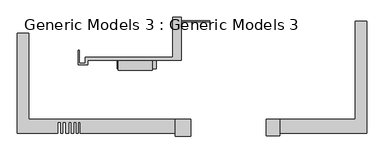
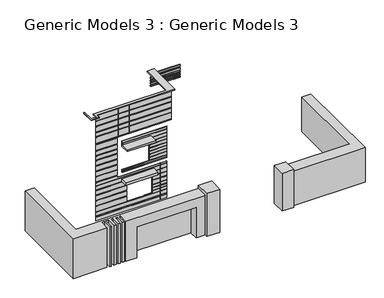
"""IFC4 building model written with IfcOpenShell, lengths in millimetres: proxy geometry, Generic Models 3 : Generic Models 3."""

from ifc_helpers import new_model, si_unit, frame, origin, place, context, project, spatial, polyline, outline, extrude, faceted_brep, source, transform, mapped, element, save


def generic_models_3_generic_models_3_b56d3d43(model_context):
    return source(origin(), model_context, "Body", "SolidModel", [
        faceted_brep([(-6055.6628107, -17805.3512614, 2871.3721498), (-6055.6628107, -17805.3512614, -304.8), (-6055.6628107, -18881.8911988, -304.8), (-6055.6628107, -18881.8911988, 2871.3721498), (-5141.2628107, -17805.3512614, 2871.3721498), (-5141.2628107, -18881.8911988, 2871.3721498), (-5141.2628107, -18881.8911988, -304.8), (-5141.2628107, -18719.7512614, -304.8), (-5141.2628107, -18719.7512614, 2606.1461296), (-5141.2628107, -17805.3512614, 2606.1461296), (-116.9337286, -17805.3512614, 2606.1461296), (-116.9337286, -17805.3512614, -304.8), (-116.9337286, -11273.8752636, -304.8), (619.6662714, -11273.8752636, -304.8), (619.6662714, -18719.7512614, -304.8), (619.6662714, -18719.7512614, 2606.1461296), (619.6662714, -11273.8752636, 2606.1461296), (-116.9337286, -11273.8752636, 2606.1461296)], [[[0, 1, 2, 3]], [[4, 5, 6, 7, 8, 9]], [[1, 0, 4, 9, 10, 11]], [[2, 1, 11, 12, 13, 14, 7, 6]], [[3, 2, 6, 5]], [[0, 3, 5, 4]], [[8, 7, 14, 15]], [[8, 15, 16, 17, 10, 9]], [[15, 14, 13, 16]], [[17, 12, 11, 10]], [[16, 13, 12, 17]]]),
        faceted_brep([(-12088.1628107, -18719.7512614, -304.8), (-12088.1628107, -18719.7512614, 3048.0), (-18387.6766205, -18719.7512614, 3048.0), (-18387.6766205, -18719.7512614, -304.8), (-17520.4293605, -18719.7512614, -304.8), (-17520.4293605, -18719.7512614, 2286.0), (-12796.0293605, -18719.7512614, 2286.0), (-12796.0293605, -18719.7512614, -304.8), (-19348.1660138, -18719.7512614, -304.8), (-19158.4539587, -18719.7512614, -304.8), (-19158.4539587, -18719.7512614, 3048.0), (-19348.1660138, -18719.7512614, 3048.0), (-18980.5989071, -18719.7512614, -304.8), (-18817.6939903, -18719.7512614, -304.8), (-18817.6939903, -18719.7512614, 3048.0), (-18980.5989071, -18719.7512614, 3048.0), (-18661.5366605, -18719.7512614, -304.8), (-18527.0628107, -18719.7512614, -304.8), (-18527.0628107, -18719.7512614, 3048.0), (-18661.5366605, -18719.7512614, 3048.0), (-19674.1502868, -18719.7512614, -304.8), (-19538.6191315, -18719.7512614, -304.8), (-19538.6191315, -18719.7512614, 3048.0), (-19674.1502868, -18719.7512614, 3048.0), (-19887.5763487, -18719.7512614, -304.8), (-19887.5763487, -18719.7512614, 3048.0), (-22558.2115964, -18719.7512614, 3048.0), (-22558.2115964, -18719.7512614, -304.8), (-21821.6115964, -17805.3512614, 3048.0), (-12088.1628107, -17805.3512614, 3048.0), (-12088.1628107, -17805.3512614, 3309.3786493), (-11046.7628107, -17805.3512614, 3309.3786493), (-11046.7628107, -17805.3512614, -304.8), (-21821.6115964, -17805.3512614, -304.8), (-11046.7628107, -18921.6642965, -304.8), (-12088.1628107, -18921.6642965, -304.8), (-12796.0293605, -17983.1512614, -304.8), (-17520.4293605, -17983.1512614, -304.8), (-18387.6766205, -17983.1512614, -304.8), (-18527.0628107, -17983.1512614, -304.8), (-18661.5366605, -17983.1512614, -304.8), (-18817.6939903, -17983.1512614, -304.8), (-18980.5989071, -17983.1512614, -304.8), (-19158.4539587, -17983.1512614, -304.8), (-19348.1660138, -17983.1512614, -304.8), (-19538.6191315, -17983.1512614, -304.8), (-19674.1502868, -17983.1512614, -304.8), (-19887.5763487, -17983.1512614, -304.8), (-22558.2115964, -12082.7142965, -304.8), (-21821.6115964, -12082.7142965, -304.8), (-21821.6115964, -12082.7142965, 3048.0), (-22558.2115964, -12082.7142965, 3048.0), (-19887.5763487, -17983.1512614, 3048.0), (-19674.1502868, -17983.1512614, 3048.0), (-19538.6191315, -17983.1512614, 3048.0), (-19348.1660138, -17983.1512614, 3048.0), (-19158.4539587, -17983.1512614, 3048.0), (-18980.5989071, -17983.1512614, 3048.0), (-18817.6939903, -17983.1512614, 3048.0), (-18661.5366605, -17983.1512614, 3048.0), (-18527.0628107, -17983.1512614, 3048.0), (-18387.6766205, -17983.1512614, 3048.0), (-11046.7628107, -18921.6642965, 3309.3786493), (-12088.1628107, -18921.6642965, 3309.3786493), (-17520.4293605, -17983.1512614, 2286.0), (-12796.0293605, -17983.1512614, 2286.0)], [[[0, 1, 2, 3, 4, 5, 6, 7]], [[8, 9, 10, 11]], [[12, 13, 14, 15]], [[16, 17, 18, 19]], [[20, 21, 22, 23]], [[24, 25, 26, 27]], [[28, 29, 30, 31, 32, 33]], [[32, 34, 35, 0, 7, 36, 37, 4, 3, 38, 39, 17, 16, 40, 41, 13, 12, 42, 43, 9, 8, 44, 45, 21, 20, 46, 47, 24, 27, 48, 49, 33]], [[29, 28, 50, 51, 26, 25, 52, 53, 23, 22, 54, 55, 11, 10, 56, 57, 15, 14, 58, 59, 19, 18, 60, 61, 2, 1]], [[62, 34, 32, 31]], [[63, 30, 29, 1, 0, 35]], [[34, 62, 63, 35]], [[62, 31, 30, 63]], [[44, 55, 54, 45]], [[42, 57, 56, 43]], [[40, 59, 58, 41]], [[38, 61, 60, 39]], [[46, 53, 52, 47]], [[45, 54, 22, 21]], [[55, 44, 8, 11]], [[43, 56, 10, 9]], [[57, 42, 12, 15]], [[41, 58, 14, 13]], [[59, 40, 16, 19]], [[39, 60, 18, 17]], [[61, 38, 3, 2]], [[47, 52, 25, 24]], [[53, 46, 20, 23]], [[64, 37, 36, 65]], [[64, 65, 6, 5]], [[65, 36, 7, 6]], [[37, 64, 5, 4]], [[51, 48, 27, 26]], [[49, 50, 28, 33]], [[48, 51, 50, 49]]]),
        faceted_brep([(-13612.1628107, -13816.2642965, 5651.3031317), (-15860.0628107, -13816.2642965, 5651.3031317), (-15860.0628107, -14540.4385796, 5651.3031317), (-13612.1628107, -14540.4385796, 5651.3031317), (-13612.1628107, -14540.4385796, 5498.9031317), (-15860.0628107, -14540.4385796, 5498.9031317), (-15860.0628107, -13816.2642965, 5498.9031317), (-13612.1628107, -13816.2642965, 5498.9031317), (-13612.1628107, -13841.6642965, 5498.9031317), (-13612.1628107, -13867.0642965, 5498.9031317)], [[[0, 1, 2, 3]], [[4, 5, 6, 7, 8, 9]], [[1, 0, 7, 6]], [[2, 1, 6, 5]], [[3, 2, 5, 4]], [[0, 3, 4, 9, 8, 7]]]),
        faceted_brep([(-15923.5628107, -13867.0642965, 2606.1461296), (-15923.5628107, -13867.0642965, 2821.2917707), (-13354.9773607, -13867.0642965, 2821.2917707), (-13354.9773607, -13867.0642965, 2606.1461296), (-12316.7628107, -13867.0642965, 2606.1461296), (-12316.7628107, -13867.0642965, 2882.1098353), (-17960.2455482, -13867.0642965, 2882.1098353), (-17960.2455482, -13867.0642965, 2606.1461296), (-12316.7628107, -13867.0642965, 3048.0), (-16279.1628107, -13867.0642965, 3048.0), (-16279.1628107, -13867.0642965, 3184.518053), (-17960.2455482, -13867.0642965, 3184.518053), (-17960.2455482, -13867.0642965, 2942.2726161), (-12316.7628107, -13867.0642965, 2942.2726161), (-17960.2455482, -13867.0642965, 0.0), (-12316.7628107, -13867.0642965, 0.0), (-12316.7628107, -13867.0642965, 304.8), (-17960.2455482, -13867.0642965, 304.8), (-11973.8628107, -13867.0642965, 8818.1896751), (-17960.2455482, -13867.0642965, 8818.1896751), (-17960.2455482, -13867.0642965, 8418.5654464), (-11973.8628107, -13867.0642965, 8418.5654464), (-15517.1628107, -13867.0642965, 2175.1008614), (-15517.1628107, -13867.0642965, 2535.4608087), (-17960.2455482, -13867.0642965, 2535.4608087), (-17960.2455482, -13867.0642965, 2175.1008614), (-15517.1628107, -13867.0642965, 1735.9125615), (-15517.1628107, -13867.0642965, 2120.9543587), (-17960.2455482, -13867.0642965, 2120.9543587), (-17960.2455482, -13867.0642965, 1735.9125615), (-15517.1628107, -13867.0642965, 763.0716334), (-15517.1628107, -13867.0642965, 1206.4800905), (-17960.2455482, -13867.0642965, 1206.4800905), (-17960.2455482, -13867.0642965, 763.0716334), (-15517.1628107, -13867.0642965, 1266.6428713), (-15517.1628107, -13867.0642965, 1684.6088815), (-17960.2455482, -13867.0642965, 1684.6088815), (-17960.2455482, -13867.0642965, 1266.6428713), (-12316.7628107, -13867.0642965, 400.2988277), (-12316.7628107, -13867.0642965, 695.0964536), (-17960.2455482, -13867.0642965, 695.0964536), (-17960.2455482, -13867.0642965, 400.2988277), (-16279.1628107, -13867.0642965, 5917.4274118), (-16279.1628107, -13867.0642965, 6400.8), (-17960.2455482, -13867.0642965, 6400.8), (-17960.2455482, -13867.0642965, 5917.4274118), (-16279.1628107, -13867.0642965, 5498.9031317), (-16279.1628107, -13867.0642965, 5825.6641304), (-17960.2455482, -13867.0642965, 5825.6641304), (-17960.2455482, -13867.0642965, 5498.9031317), (-16279.1628107, -13867.0642965, 5103.7107607), (-16279.1628107, -13867.0642965, 5410.5409428), (-17960.2455482, -13867.0642965, 5410.5409428), (-17960.2455482, -13867.0642965, 5103.7107607), (-16279.1628107, -13867.0642965, 4670.5387389), (-16279.1628107, -13867.0642965, 5043.5479799), (-17960.2455482, -13867.0642965, 5043.5479799), (-17960.2455482, -13867.0642965, 4670.5387389), (-16279.1628107, -13867.0642965, 4207.2853267), (-16279.1628107, -13867.0642965, 4598.343402), (-17960.2455482, -13867.0642965, 4598.343402), (-17960.2455482, -13867.0642965, 4207.2853267), (-16279.1628107, -13867.0642965, 3750.0481926), (-16279.1628107, -13867.0642965, 4124.9991955), (-17960.2455482, -13867.0642965, 4124.9991955), (-17960.2455482, -13867.0642965, 3750.0481926), (-16279.1628107, -13867.0642965, 3256.71339), (-16279.1628107, -13867.0642965, 3701.917968), (-17960.2455482, -13867.0642965, 3701.917968), (-17960.2455482, -13867.0642965, 3256.71339), (-11973.8628107, -13867.0642965, 7978.3125268), (-11973.8628107, -13867.0642965, 8337.4712494), (-17960.2455482, -13867.0642965, 8337.4712494), (-17960.2455482, -13867.0642965, 7978.3125268), (-11973.8628107, -13867.0642965, 7494.0021413), (-11973.8628107, -13867.0642965, 7895.2878893), (-17960.2455482, -13867.0642965, 7895.2878893), (-17960.2455482, -13867.0642965, 7494.0021413), (-11973.8628107, -13867.0642965, 7078.8789538), (-11973.8628107, -13867.0642965, 7410.9775038), (-17960.2455482, -13867.0642965, 7410.9775038), (-17960.2455482, -13867.0642965, 7078.8789538), (-11973.8628107, -13867.0642965, 6495.9664367), (-11973.8628107, -13867.0642965, 7011.586349), (-17960.2455482, -13867.0642965, 7011.586349), (-17960.2455482, -13867.0642965, 6495.9664367), (-13497.8628107, -13867.0642965, 763.0716334), (-12316.7628107, -13867.0642965, 763.0716334), (-12316.7628107, -13867.0642965, 953.616846), (-13497.8628107, -13867.0642965, 953.616846), (-13497.8628107, -13867.0642965, 2540.7233827), (-13497.8628107, -13867.0642965, 2245.0272955), (-12316.7628107, -13867.0642965, 2245.0272955), (-12316.7628107, -13867.0642965, 2540.7233827), (-13497.8628107, -13867.0642965, 2176.789737), (-13497.8628107, -13867.0642965, 1876.5444793), (-12316.7628107, -13867.0642965, 1876.5444793), (-12316.7628107, -13867.0642965, 2176.789737), (-13497.8628107, -13867.0642965, 1822.5907344), (-13497.8628107, -13867.0642965, 1524.0), (-12316.7628107, -13867.0642965, 1524.0), (-12316.7628107, -13867.0642965, 1822.5907344), (-13497.8628107, -13867.0642965, 1462.5699573), (-13497.8628107, -13867.0642965, 1249.7277266), (-12316.7628107, -13867.0642965, 1249.7277266), (-12316.7628107, -13867.0642965, 1462.5699573), (-13497.8628107, -13867.0642965, 1194.1688936), (-13497.8628107, -13867.0642965, 1001.3322189), (-12316.7628107, -13867.0642965, 1001.3322189), (-12316.7628107, -13867.0642965, 1194.1688936), (-15923.5628107, -13816.2642965, 2606.1461296), (-15517.1628107, -13816.2642965, 2606.1461296), (-15517.1628107, -13816.2642965, 0.0), (-16170.5880908, -13816.2642965, 0.0), (-16170.5880908, -13816.2642965, 3048.0), (-12953.063671, -13816.2642965, 3048.0), (-12953.063671, -13816.2642965, 0.0), (-13497.8628107, -13816.2642965, 0.0), (-13497.8628107, -13816.2642965, 2606.1461296), (-13354.9773607, -13816.2642965, 2606.1461296), (-13354.9773607, -13816.2642965, 2821.2917707), (-15923.5628107, -13816.2642965, 2821.2917707), (-12316.7628107, -13816.2642965, 3048.0), (-12316.7628107, -13816.2642965, 0.0), (-12850.1628107, -13816.2642965, 0.0), (-12850.1628107, -13816.2642965, 3048.0), (-11973.8628107, -13816.2642965, 8818.1896751), (-11973.8628107, -13816.2642965, 6400.8), (-12768.5357054, -13816.2642965, 6400.8), (-12768.5357054, -13816.2642965, 8818.1896751), (-17960.2455482, -13816.2642965, 0.0), (-17960.2455482, -13816.2642965, 8818.1896751), (-17079.2628107, -13816.2642965, 8818.1896751), (-17079.2628107, -13816.2642965, 0.0), (-16279.1628107, -13816.2642965, 0.0), (-16980.0783065, -13816.2642965, 0.0), (-16980.0783065, -13816.2642965, 8818.1896751), (-16279.1628107, -13816.2642965, 8818.1896751), (-14673.1364765, -13816.2642965, 0.0), (-15421.9128107, -13816.2642965, 0.0), (-15421.9128107, -13816.2642965, 763.0716334), (-14673.1364765, -13816.2642965, 763.0716334), (-13565.9475269, -13816.2642965, 0.0), (-14032.5674721, -13816.2642965, 0.0), (-14032.5674721, -13816.2642965, 763.0716334), (-13565.9475269, -13816.2642965, 763.0716334), (-14071.4524675, -13816.2642965, 0.0), (-14564.6628107, -13816.2642965, 0.0), (-14564.6628107, -13816.2642965, 763.0716334), (-14071.4524675, -13816.2642965, 763.0716334), (-16187.9466003, -13816.2642965, 8818.1896751), (-15402.8628107, -13816.2642965, 8818.1896751), (-15402.8628107, -13816.2642965, 6495.9664367), (-15312.895459, -13816.2642965, 6495.9664367), (-15312.895459, -13816.2642965, 8818.1896751), (-14567.4028515, -13816.2642965, 8818.1896751), (-14567.4028515, -13816.2642965, 6400.8), (-16187.9466003, -13816.2642965, 6400.8), (-14463.6220546, -13816.2642965, 8818.1896751), (-13726.4628107, -13816.2642965, 8818.1896751), (-13726.4628107, -13816.2642965, 6400.8), (-14463.6220546, -13816.2642965, 6400.8), (-13612.1628107, -13816.2642965, 8818.1896751), (-12879.2352221, -13816.2642965, 8818.1896751), (-12879.2352221, -13816.2642965, 6400.8), (-13612.1628107, -13816.2642965, 6400.8), (-17960.2455482, -13841.6642965, 304.8), (-17960.2455482, -13841.6642965, 400.2988277), (-17960.2455482, -13841.6642965, 695.0964536), (-17960.2455482, -13841.6642965, 763.0716334), (-17960.2455482, -13841.6642965, 1206.4800905), (-17960.2455482, -13841.6642965, 1266.6428713), (-17960.2455482, -13841.6642965, 1684.6088815), (-17960.2455482, -13841.6642965, 1735.9125615), (-17960.2455482, -13841.6642965, 2120.9543587), (-17960.2455482, -13841.6642965, 2175.1008614), (-17960.2455482, -13841.6642965, 2535.4608087), (-17960.2455482, -13841.6642965, 2606.1461296), (-17960.2455482, -13841.6642965, 2882.1098353), (-17960.2455482, -13841.6642965, 2942.2726161), (-17960.2455482, -13841.6642965, 3184.518053), (-17960.2455482, -13841.6642965, 3256.71339), (-17960.2455482, -13841.6642965, 3701.917968), (-17960.2455482, -13841.6642965, 3750.0481926), (-17960.2455482, -13841.6642965, 4124.9991955), (-17960.2455482, -13841.6642965, 4207.2853267), (-17960.2455482, -13841.6642965, 4598.343402), (-17960.2455482, -13841.6642965, 4670.5387389), (-17960.2455482, -13841.6642965, 5043.5479799), (-17960.2455482, -13841.6642965, 5103.7107607), (-17960.2455482, -13841.6642965, 5410.5409428), (-17960.2455482, -13841.6642965, 5498.9031317), (-17960.2455482, -13841.6642965, 5825.6641304), (-17960.2455482, -13841.6642965, 5917.4274118), (-17960.2455482, -13841.6642965, 6400.8), (-17960.2455482, -13841.6642965, 6495.9664367), (-17960.2455482, -13841.6642965, 7011.586349), (-17960.2455482, -13841.6642965, 7078.8789538), (-17960.2455482, -13841.6642965, 7410.9775038), (-17960.2455482, -13841.6642965, 7494.0021413), (-17960.2455482, -13841.6642965, 7895.2878893), (-17960.2455482, -13841.6642965, 7978.3125268), (-17960.2455482, -13841.6642965, 8337.4712494), (-17960.2455482, -13841.6642965, 8418.5654464), (-17079.2628107, -13841.6642965, 0.0), (-16980.0783065, -13841.6642965, 0.0), (-16279.1628107, -13841.6642965, 0.0), (-16170.5880908, -13841.6642965, 0.0), (-15517.1628107, -13841.6642965, 0.0), (-15421.9128107, -13841.6642965, 0.0), (-14673.1364765, -13841.6642965, 0.0), (-14564.6628107, -13841.6642965, 0.0), (-14071.4524675, -13841.6642965, 0.0), (-14032.5674721, -13841.6642965, 0.0), (-13565.9475269, -13841.6642965, 0.0), (-13497.8628107, -13841.6642965, 0.0), (-12953.063671, -13841.6642965, 0.0), (-12850.1628107, -13841.6642965, 0.0), (-16279.1628107, -13841.6642965, 5917.4274118), (-16279.1628107, -13841.6642965, 5825.6641304), (-16279.1628107, -13841.6642965, 5498.9031317), (-16279.1628107, -13841.6642965, 5410.5409428), (-16279.1628107, -13841.6642965, 5103.7107607), (-16279.1628107, -13841.6642965, 5043.5479799), (-16279.1628107, -13841.6642965, 4670.5387389), (-16279.1628107, -13841.6642965, 4598.343402), (-16279.1628107, -13841.6642965, 4207.2853267), (-16279.1628107, -13841.6642965, 4124.9991955), (-16279.1628107, -13841.6642965, 3750.0481926), (-16279.1628107, -13841.6642965, 3701.917968), (-16279.1628107, -13841.6642965, 3256.71339), (-16279.1628107, -13841.6642965, 3184.518053), (-16279.1628107, -13841.6642965, 3048.0), (-16279.1628107, -13841.6642965, 2942.2726161), (-16279.1628107, -13841.6642965, 2882.1098353), (-16279.1628107, -13841.6642965, 2606.1461296), (-16279.1628107, -13841.6642965, 2535.4608087), (-16279.1628107, -13841.6642965, 2175.1008614), (-16279.1628107, -13841.6642965, 2120.9543587), (-16279.1628107, -13841.6642965, 1735.9125615), (-16279.1628107, -13841.6642965, 1684.6088815), (-16279.1628107, -13841.6642965, 1266.6428713), (-16279.1628107, -13841.6642965, 1206.4800905), (-16279.1628107, -13841.6642965, 763.0716334), (-16279.1628107, -13841.6642965, 695.0964536), (-16279.1628107, -13841.6642965, 400.2988277), (-16279.1628107, -13841.6642965, 304.8), (-16279.1628107, -13841.6642965, 8818.1896751), (-16279.1628107, -13841.6642965, 8418.5654464), (-16279.1628107, -13841.6642965, 8337.4712494), (-16279.1628107, -13841.6642965, 7978.3125268), (-16279.1628107, -13841.6642965, 7895.2878893), (-16279.1628107, -13841.6642965, 7494.0021413), (-16279.1628107, -13841.6642965, 7410.9775038), (-16279.1628107, -13841.6642965, 7078.8789538), (-16279.1628107, -13841.6642965, 7011.586349), (-16279.1628107, -13841.6642965, 6495.9664367), (-16279.1628107, -13841.6642965, 6400.8), (-12850.1628107, -13841.6642965, 3048.0), (-12953.063671, -13841.6642965, 3048.0), (-16170.5880908, -13841.6642965, 3048.0), (-15517.1628107, -13841.6642965, 2175.1008614), (-15517.1628107, -13841.6642965, 2120.9543587), (-15517.1628107, -13841.6642965, 1735.9125615), (-15517.1628107, -13841.6642965, 1684.6088815), (-15517.1628107, -13841.6642965, 1266.6428713), (-15517.1628107, -13841.6642965, 1206.4800905), (-15517.1628107, -13841.6642965, 763.0716334), (-15517.1628107, -13841.6642965, 695.0964536), (-15517.1628107, -13841.6642965, 400.2988277), (-15517.1628107, -13841.6642965, 304.8), (-15517.1628107, -13841.6642965, 2606.1461296), (-15517.1628107, -13841.6642965, 2535.4608087), (-13354.9773607, -13701.9642965, 2821.2917707), (-15923.5628107, -13701.9642965, 2821.2917707), (-15923.5628107, -14431.1224926, 2821.2917707), (-13354.9773607, -14431.1224926, 2821.2917707), (-13354.9773607, -14431.1224926, 2606.1461296), (-15923.5628107, -14431.1224926, 2606.1461296), (-17079.2628107, -13841.6642965, 2606.1461296), (-16980.0783065, -13841.6642965, 2606.1461296), (-16170.5880908, -13841.6642965, 2606.1461296), (-15923.5628107, -13701.9642965, 2606.1461296), (-13354.9773607, -13701.9642965, 2606.1461296), (-13497.8628107, -13841.6642965, 2606.1461296), (-12953.063671, -13841.6642965, 2606.1461296), (-12850.1628107, -13841.6642965, 2606.1461296), (-12316.7628107, -13841.6642965, 2606.1461296), (-12316.7628107, -13841.6642965, 2942.2726161), (-12316.7628107, -13841.6642965, 2882.1098353), (-12316.7628107, -13841.6642965, 2540.7233827), (-12316.7628107, -13841.6642965, 2245.0272955), (-12316.7628107, -13841.6642965, 2176.789737), (-12316.7628107, -13841.6642965, 1876.5444793), (-12316.7628107, -13841.6642965, 1822.5907344), (-12316.7628107, -13841.6642965, 1524.0), (-12316.7628107, -13841.6642965, 1462.5699573), (-12316.7628107, -13841.6642965, 1249.7277266), (-12316.7628107, -13841.6642965, 1194.1688936), (-12316.7628107, -13841.6642965, 1001.3322189), (-12316.7628107, -13841.6642965, 953.616846), (-12316.7628107, -13841.6642965, 763.0716334), (-12316.7628107, -13841.6642965, 695.0964536), (-12316.7628107, -13841.6642965, 400.2988277), (-12316.7628107, -13841.6642965, 304.8), (-13497.8628107, -13841.6642965, 763.0716334), (-13497.8628107, -13841.6642965, 953.616846), (-13497.8628107, -13841.6642965, 1001.3322189), (-13497.8628107, -13841.6642965, 1194.1688936), (-13497.8628107, -13841.6642965, 1249.7277266), (-13497.8628107, -13841.6642965, 1462.5699573), (-13497.8628107, -13841.6642965, 1524.0), (-13497.8628107, -13841.6642965, 1822.5907344), (-13497.8628107, -13841.6642965, 1876.5444793), (-13497.8628107, -13841.6642965, 2176.789737), (-13497.8628107, -13841.6642965, 2245.0272955), (-13497.8628107, -13841.6642965, 2540.7233827), (-13497.8628107, -13841.6642965, 304.8), (-13497.8628107, -13841.6642965, 400.2988277), (-13497.8628107, -13841.6642965, 695.0964536), (-15421.9128107, -13841.6642965, 763.0716334), (-14673.1364765, -13841.6642965, 763.0716334), (-14032.5674721, -13841.6642965, 763.0716334), (-13565.9475269, -13841.6642965, 763.0716334), (-14564.6628107, -13841.6642965, 763.0716334), (-14071.4524675, -13841.6642965, 763.0716334), (-11973.8628107, -13841.6642965, 8418.5654464), (-11973.8628107, -13841.6642965, 8337.4712494), (-11973.8628107, -13841.6642965, 7978.3125268), (-11973.8628107, -13841.6642965, 7895.2878893), (-11973.8628107, -13841.6642965, 7494.0021413), (-11973.8628107, -13841.6642965, 7410.9775038), (-11973.8628107, -13841.6642965, 7078.8789538), (-11973.8628107, -13841.6642965, 7011.586349), (-11973.8628107, -13841.6642965, 6495.9664367), (-11973.8628107, -13841.6642965, 6400.8), (-12768.5357054, -13841.6642965, 8818.1896751), (-12879.2352221, -13841.6642965, 8818.1896751), (-13612.1628107, -13841.6642965, 8818.1896751), (-13726.4628107, -13841.6642965, 8818.1896751), (-14463.6220546, -13841.6642965, 8818.1896751), (-14567.4028515, -13841.6642965, 8818.1896751), (-15312.895459, -13841.6642965, 8818.1896751), (-15402.8628107, -13841.6642965, 8818.1896751), (-16187.9466003, -13841.6642965, 8818.1896751), (-16980.0783065, -13841.6642965, 8818.1896751), (-17079.2628107, -13841.6642965, 8818.1896751), (-14567.4028515, -13841.6642965, 6400.8), (-16187.9466003, -13841.6642965, 6400.8), (-13726.4628107, -13841.6642965, 6400.8), (-14463.6220546, -13841.6642965, 6400.8), (-12879.2352221, -13841.6642965, 6400.8), (-13612.1628107, -13841.6642965, 6400.8), (-12768.5357054, -13841.6642965, 6400.8), (-17079.2628107, -13841.6642965, 304.8), (-17079.2628107, -13841.6642965, 400.2988277), (-17079.2628107, -13841.6642965, 695.0964536), (-17079.2628107, -13841.6642965, 763.0716334), (-17079.2628107, -13841.6642965, 1206.4800905), (-17079.2628107, -13841.6642965, 1266.6428713), (-17079.2628107, -13841.6642965, 1684.6088815), (-17079.2628107, -13841.6642965, 1735.9125615), (-17079.2628107, -13841.6642965, 2120.9543587), (-17079.2628107, -13841.6642965, 2175.1008614), (-17079.2628107, -13841.6642965, 2535.4608087), (-17079.2628107, -13841.6642965, 2882.1098353), (-17079.2628107, -13841.6642965, 2942.2726161), (-17079.2628107, -13841.6642965, 3184.518053), (-17079.2628107, -13841.6642965, 3256.71339), (-17079.2628107, -13841.6642965, 3701.917968), (-17079.2628107, -13841.6642965, 3750.0481926), (-17079.2628107, -13841.6642965, 4124.9991955), (-17079.2628107, -13841.6642965, 4207.2853267), (-17079.2628107, -13841.6642965, 4598.343402), (-17079.2628107, -13841.6642965, 4670.5387389), (-17079.2628107, -13841.6642965, 5043.5479799), (-17079.2628107, -13841.6642965, 5103.7107607), (-17079.2628107, -13841.6642965, 5410.5409428), (-17079.2628107, -13841.6642965, 5498.9031317), (-17079.2628107, -13841.6642965, 5825.6641304), (-17079.2628107, -13841.6642965, 5917.4274118), (-17079.2628107, -13841.6642965, 6400.8), (-17079.2628107, -13841.6642965, 6495.9664367), (-17079.2628107, -13841.6642965, 7011.586349), (-17079.2628107, -13841.6642965, 7078.8789538), (-17079.2628107, -13841.6642965, 7410.9775038), (-17079.2628107, -13841.6642965, 7494.0021413), (-17079.2628107, -13841.6642965, 7895.2878893), (-17079.2628107, -13841.6642965, 7978.3125268), (-17079.2628107, -13841.6642965, 8337.4712494), (-17079.2628107, -13841.6642965, 8418.5654464), (-16980.0783065, -13841.6642965, 5917.4274118), (-16980.0783065, -13841.6642965, 5825.6641304), (-16980.0783065, -13841.6642965, 5498.9031317), (-16980.0783065, -13841.6642965, 5410.5409428), (-16980.0783065, -13841.6642965, 5103.7107607), (-16980.0783065, -13841.6642965, 5043.5479799), (-16980.0783065, -13841.6642965, 4670.5387389), (-16980.0783065, -13841.6642965, 4598.343402), (-16980.0783065, -13841.6642965, 4207.2853267), (-16980.0783065, -13841.6642965, 4124.9991955), (-16980.0783065, -13841.6642965, 3750.0481926), (-16980.0783065, -13841.6642965, 3701.917968), (-16980.0783065, -13841.6642965, 3256.71339), (-16980.0783065, -13841.6642965, 3184.518053), (-16170.5880908, -13841.6642965, 2175.1008614), (-16170.5880908, -13841.6642965, 2120.9543587), (-16170.5880908, -13841.6642965, 1735.9125615), (-16170.5880908, -13841.6642965, 1684.6088815), (-16170.5880908, -13841.6642965, 1266.6428713), (-16170.5880908, -13841.6642965, 1206.4800905), (-16170.5880908, -13841.6642965, 2535.4608087), (-16980.0783065, -13841.6642965, 2535.4608087), (-12850.1628107, -13841.6642965, 2942.2726161), (-12850.1628107, -13841.6642965, 2882.1098353), (-12850.1628107, -13841.6642965, 763.0716334), (-12850.1628107, -13841.6642965, 695.0964536), (-12850.1628107, -13841.6642965, 400.2988277), (-12850.1628107, -13841.6642965, 304.8), (-15421.9128107, -13841.6642965, 695.0964536), (-14673.1364765, -13841.6642965, 695.0964536), (-14032.5674721, -13841.6642965, 695.0964536), (-13565.9475269, -13841.6642965, 695.0964536), (-14564.6628107, -13841.6642965, 695.0964536), (-14071.4524675, -13841.6642965, 695.0964536), (-12768.5357054, -13841.6642965, 8418.5654464), (-12768.5357054, -13841.6642965, 8337.4712494), (-12768.5357054, -13841.6642965, 7978.3125268), (-12768.5357054, -13841.6642965, 7895.2878893), (-12768.5357054, -13841.6642965, 7494.0021413), (-12768.5357054, -13841.6642965, 7410.9775038), (-12768.5357054, -13841.6642965, 7078.8789538), (-12768.5357054, -13841.6642965, 7011.586349), (-12768.5357054, -13841.6642965, 6495.9664367), (-14567.4028515, -13841.6642965, 6495.9664367), (-15312.895459, -13841.6642965, 6495.9664367), (-15402.8628107, -13841.6642965, 6495.9664367), (-16187.9466003, -13841.6642965, 6495.9664367), (-13726.4628107, -13841.6642965, 6495.9664367), (-14463.6220546, -13841.6642965, 6495.9664367), (-12879.2352221, -13841.6642965, 6495.9664367), (-13612.1628107, -13841.6642965, 6495.9664367), (-15402.8628107, -13841.6642965, 8418.5654464), (-16187.9466003, -13841.6642965, 8418.5654464), (-16187.9466003, -13841.6642965, 8337.4712494), (-15402.8628107, -13841.6642965, 8337.4712494), (-14567.4028515, -13841.6642965, 8418.5654464), (-15312.895459, -13841.6642965, 8418.5654464), (-15312.895459, -13841.6642965, 8337.4712494), (-14567.4028515, -13841.6642965, 8337.4712494), (-13726.4628107, -13841.6642965, 8418.5654464), (-14463.6220546, -13841.6642965, 8418.5654464), (-14463.6220546, -13841.6642965, 8337.4712494), (-13726.4628107, -13841.6642965, 8337.4712494), (-12879.2352221, -13841.6642965, 8418.5654464), (-13612.1628107, -13841.6642965, 8418.5654464), (-13612.1628107, -13841.6642965, 8337.4712494), (-12879.2352221, -13841.6642965, 8337.4712494), (-16980.0783065, -13841.6642965, 8418.5654464), (-16980.0783065, -13841.6642965, 8337.4712494), (-15402.8628107, -13841.6642965, 7978.3125268), (-16187.9466003, -13841.6642965, 7978.3125268), (-16187.9466003, -13841.6642965, 7895.2878893), (-15402.8628107, -13841.6642965, 7895.2878893), (-14567.4028515, -13841.6642965, 7978.3125268), (-15312.895459, -13841.6642965, 7978.3125268), (-15312.895459, -13841.6642965, 7895.2878893), (-14567.4028515, -13841.6642965, 7895.2878893), (-13726.4628107, -13841.6642965, 7978.3125268), (-14463.6220546, -13841.6642965, 7978.3125268), (-14463.6220546, -13841.6642965, 7895.2878893), (-13726.4628107, -13841.6642965, 7895.2878893), (-12879.2352221, -13841.6642965, 7978.3125268), (-13612.1628107, -13841.6642965, 7978.3125268), (-13612.1628107, -13841.6642965, 7895.2878893), (-12879.2352221, -13841.6642965, 7895.2878893), (-16980.0783065, -13841.6642965, 7978.3125268), (-16980.0783065, -13841.6642965, 7895.2878893), (-15402.8628107, -13841.6642965, 7494.0021413), (-16187.9466003, -13841.6642965, 7494.0021413), (-16187.9466003, -13841.6642965, 7410.9775038), (-15402.8628107, -13841.6642965, 7410.9775038), (-14567.4028515, -13841.6642965, 7494.0021413), (-15312.895459, -13841.6642965, 7494.0021413), (-15312.895459, -13841.6642965, 7410.9775038), (-14567.4028515, -13841.6642965, 7410.9775038), (-13726.4628107, -13841.6642965, 7494.0021413), (-14463.6220546, -13841.6642965, 7494.0021413), (-14463.6220546, -13841.6642965, 7410.9775038), (-13726.4628107, -13841.6642965, 7410.9775038), (-12879.2352221, -13841.6642965, 7494.0021413), (-13612.1628107, -13841.6642965, 7494.0021413), (-13612.1628107, -13841.6642965, 7410.9775038), (-12879.2352221, -13841.6642965, 7410.9775038), (-16980.0783065, -13841.6642965, 7494.0021413), (-16980.0783065, -13841.6642965, 7410.9775038), (-15402.8628107, -13841.6642965, 7078.8789538), (-16187.9466003, -13841.6642965, 7078.8789538), (-16187.9466003, -13841.6642965, 7011.586349), (-15402.8628107, -13841.6642965, 7011.586349), (-14567.4028515, -13841.6642965, 7078.8789538), (-15312.895459, -13841.6642965, 7078.8789538), (-15312.895459, -13841.6642965, 7011.586349), (-14567.4028515, -13841.6642965, 7011.586349), (-13726.4628107, -13841.6642965, 7078.8789538), (-14463.6220546, -13841.6642965, 7078.8789538), (-14463.6220546, -13841.6642965, 7011.586349), (-13726.4628107, -13841.6642965, 7011.586349), (-12879.2352221, -13841.6642965, 7078.8789538), (-13612.1628107, -13841.6642965, 7078.8789538), (-13612.1628107, -13841.6642965, 7011.586349), (-12879.2352221, -13841.6642965, 7011.586349), (-16980.0783065, -13841.6642965, 7078.8789538), (-16980.0783065, -13841.6642965, 7011.586349), (-16980.0783065, -13841.6642965, 6495.9664367), (-16980.0783065, -13841.6642965, 6400.8), (-16980.0783065, -13841.6642965, 2942.2726161), (-16980.0783065, -13841.6642965, 2882.1098353), (-12953.063671, -13841.6642965, 2942.2726161), (-16170.5880908, -13841.6642965, 2942.2726161), (-16170.5880908, -13841.6642965, 2882.1098353), (-12953.063671, -13841.6642965, 2882.1098353), (-16980.0783065, -13841.6642965, 2175.1008614), (-16980.0783065, -13841.6642965, 2120.9543587), (-16980.0783065, -13841.6642965, 1735.9125615), (-16980.0783065, -13841.6642965, 1684.6088815), (-16980.0783065, -13841.6642965, 1266.6428713), (-16980.0783065, -13841.6642965, 1206.4800905), (-16980.0783065, -13841.6642965, 695.0964536), (-16980.0783065, -13841.6642965, 763.0716334), (-16170.5880908, -13841.6642965, 695.0964536), (-16170.5880908, -13841.6642965, 763.0716334), (-12953.063671, -13841.6642965, 695.0964536), (-12953.063671, -13841.6642965, 763.0716334), (-16980.0783065, -13841.6642965, 400.2988277), (-16980.0783065, -13841.6642965, 304.8), (-16170.5880908, -13841.6642965, 400.2988277), (-16170.5880908, -13841.6642965, 304.8), (-14673.1364765, -13841.6642965, 400.2988277), (-15421.9128107, -13841.6642965, 400.2988277), (-15421.9128107, -13841.6642965, 304.8), (-14673.1364765, -13841.6642965, 304.8), (-13565.9475269, -13841.6642965, 400.2988277), (-14032.5674721, -13841.6642965, 400.2988277), (-14032.5674721, -13841.6642965, 304.8), (-13565.9475269, -13841.6642965, 304.8), (-14071.4524675, -13841.6642965, 400.2988277), (-14564.6628107, -13841.6642965, 400.2988277), (-14564.6628107, -13841.6642965, 304.8), (-14071.4524675, -13841.6642965, 304.8), (-12953.063671, -13841.6642965, 400.2988277), (-12953.063671, -13841.6642965, 304.8), (-12953.063671, -13841.6642965, 953.616846), (-12850.1628107, -13841.6642965, 953.616846), (-15312.895459, -13841.6642965, 6495.9664367), (-15402.8628107, -13841.6642965, 6495.9664367), (-12850.1628107, -13841.6642965, 2540.7233827), (-12850.1628107, -13841.6642965, 2245.0272955), (-12953.063671, -13841.6642965, 2245.0272955), (-12953.063671, -13841.6642965, 2540.7233827), (-12850.1628107, -13841.6642965, 2176.789737), (-12850.1628107, -13841.6642965, 1876.5444793), (-12953.063671, -13841.6642965, 1876.5444793), (-12953.063671, -13841.6642965, 2176.789737), (-12850.1628107, -13841.6642965, 1822.5907344), (-12850.1628107, -13841.6642965, 1524.0), (-12953.063671, -13841.6642965, 1524.0), (-12953.063671, -13841.6642965, 1822.5907344), (-12850.1628107, -13841.6642965, 1462.5699573), (-12850.1628107, -13841.6642965, 1249.7277266), (-12953.063671, -13841.6642965, 1249.7277266), (-12953.063671, -13841.6642965, 1462.5699573), (-12850.1628107, -13841.6642965, 1194.1688936), (-12850.1628107, -13841.6642965, 1001.3322189), (-12953.063671, -13841.6642965, 1001.3322189), (-12953.063671, -13841.6642965, 1194.1688936)], [[[0, 1, 2, 3, 4, 5, 6, 7]], [[8, 9, 10, 11, 12, 13]], [[14, 15, 16, 17]], [[18, 19, 20, 21]], [[22, 23, 24, 25]], [[26, 27, 28, 29]], [[30, 31, 32, 33]], [[34, 35, 36, 37]], [[38, 39, 40, 41]], [[42, 43, 44, 45]], [[46, 47, 48, 49]], [[50, 51, 52, 53]], [[54, 55, 56, 57]], [[58, 59, 60, 61]], [[62, 63, 64, 65]], [[66, 67, 68, 69]], [[70, 71, 72, 73]], [[74, 75, 76, 77]], [[78, 79, 80, 81]], [[82, 83, 84, 85]], [[86, 87, 88, 89]], [[90, 91, 92, 93]], [[94, 95, 96, 97]], [[98, 99, 100, 101]], [[102, 103, 104, 105]], [[106, 107, 108, 109]], [[110, 111, 112, 113, 114, 115, 116, 117, 118, 119, 120, 121]], [[122, 123, 124, 125]], [[126, 127, 128, 129]], [[130, 131, 132, 133]], [[134, 135, 136, 137]], [[138, 139, 140, 141]], [[142, 143, 144, 145]], [[146, 147, 148, 149]], [[150, 151, 152, 153, 154, 155, 156, 157]], [[158, 159, 160, 161]], [[162, 163, 164, 165]], [[130, 14, 17, 166, 167, 41, 40, 168, 169, 33, 32, 170, 171, 37, 36, 172, 173, 29, 28, 174, 175, 25, 24, 176, 177, 7, 6, 178, 179, 12, 11, 180, 181, 69, 68, 182, 183, 65, 64, 184, 185, 61, 60, 186, 187, 57, 56, 188, 189, 53, 52, 190, 191, 49, 48, 192, 193, 45, 44, 194, 195, 85, 84, 196, 197, 81, 80, 198, 199, 77, 76, 200, 201, 73, 72, 202, 203, 20, 19, 131]], [[14, 130, 133, 204, 205, 135, 134, 206, 207, 113, 112, 208, 209, 139, 138, 210, 211, 147, 146, 212, 213, 143, 142, 214, 215, 117, 116, 216, 217, 124, 123, 15]], [[43, 42, 218, 219, 47, 46, 220, 221, 51, 50, 222, 223, 55, 54, 224, 225, 59, 58, 226, 227, 63, 62, 228, 229, 67, 66, 230, 231, 10, 9, 232, 233, 234, 235, 236, 237, 238, 239, 240, 241, 242, 243, 244, 245, 246, 206, 134, 137, 247, 248, 249, 250, 251, 252, 253, 254, 255, 256, 257]], [[8, 122, 125, 258, 259, 115, 114, 260, 232, 9]], [[23, 22, 261, 262, 27, 26, 263, 264, 35, 34, 265, 266, 31, 30, 267, 268, 269, 270, 208, 112, 111, 271, 272]], [[273, 274, 121, 120]], [[275, 276, 2, 1]], [[277, 278, 0, 7, 177, 279, 280, 235, 281, 271, 111, 110, 282, 283, 119, 118, 284, 285, 286, 287, 4, 3]], [[274, 273, 283, 282]], [[274, 282, 110, 121]], [[278, 275, 1, 0]], [[276, 275, 278, 277]], [[283, 273, 120, 119]], [[276, 277, 3, 2]], [[122, 8, 13, 288, 289, 5, 4, 287, 290, 93, 92, 291, 292, 97, 96, 293, 294, 101, 100, 295, 296, 105, 104, 297, 298, 109, 108, 299, 300, 88, 87, 301, 302, 39, 38, 303, 304, 16, 15, 123]], [[305, 86, 89, 306, 307, 107, 106, 308, 309, 103, 102, 310, 311, 99, 98, 312, 313, 95, 94, 314, 315, 91, 90, 316, 284, 118, 117, 215, 317, 318, 319]], [[141, 140, 320, 321]], [[145, 144, 322, 323]], [[149, 148, 324, 325]], [[127, 126, 18, 21, 326, 327, 71, 70, 328, 329, 75, 74, 330, 331, 79, 78, 332, 333, 83, 82, 334, 335]], [[19, 18, 126, 129, 336, 337, 163, 162, 338, 339, 159, 158, 340, 341, 155, 154, 342, 343, 151, 150, 344, 247, 137, 136, 345, 346, 132, 131]], [[157, 156, 347, 348]], [[161, 160, 349, 350]], [[165, 164, 351, 352]], [[127, 335, 353, 128]], [[167, 166, 354, 355]], [[169, 168, 356, 357]], [[171, 170, 358, 359]], [[173, 172, 360, 361]], [[175, 174, 362, 363]], [[177, 176, 364, 279]], [[179, 178, 365, 366]], [[181, 180, 367, 368]], [[183, 182, 369, 370]], [[185, 184, 371, 372]], [[187, 186, 373, 374]], [[189, 188, 375, 376]], [[191, 190, 377, 378]], [[193, 192, 379, 380]], [[195, 194, 381, 382]], [[197, 196, 383, 384]], [[199, 198, 385, 386]], [[201, 200, 387, 388]], [[203, 202, 389, 390]], [[219, 218, 391, 392]], [[221, 220, 393, 394]], [[223, 222, 395, 396]], [[225, 224, 397, 398]], [[227, 226, 399, 400]], [[229, 228, 401, 402]], [[231, 230, 403, 404]], [[262, 261, 405, 406]], [[264, 263, 407, 408]], [[266, 265, 409, 410]], [[272, 271, 281, 411]], [[235, 280, 412, 236]], [[289, 288, 413, 414]], [[302, 301, 415, 416]], [[304, 303, 417, 418]], [[321, 320, 419, 420]], [[323, 322, 421, 422]], [[325, 324, 423, 424]], [[327, 326, 425, 426]], [[329, 328, 427, 428]], [[331, 330, 429, 430]], [[333, 332, 431, 432]], [[335, 334, 433, 353]], [[348, 347, 434, 435, 436, 437]], [[350, 349, 438, 439]], [[352, 351, 440, 441]], [[442, 443, 444, 445]], [[446, 447, 448, 449]], [[450, 451, 452, 453]], [[454, 455, 456, 457]], [[248, 458, 459, 249]], [[460, 461, 462, 463]], [[464, 465, 466, 467]], [[468, 469, 470, 471]], [[472, 473, 474, 475]], [[250, 476, 477, 251]], [[478, 479, 480, 481]], [[482, 483, 484, 485]], [[486, 487, 488, 489]], [[490, 491, 492, 493]], [[252, 494, 495, 253]], [[496, 497, 498, 499]], [[500, 501, 502, 503]], [[504, 505, 506, 507]], [[508, 509, 510, 511]], [[254, 512, 513, 255]], [[256, 514, 515, 257]], [[233, 516, 517, 234]], [[518, 519, 520, 521]], [[237, 522, 523, 238]], [[239, 524, 525, 240]], [[241, 526, 527, 242]], [[528, 244, 243, 529]], [[530, 268, 267, 531]], [[319, 532, 533, 305]], [[245, 534, 535, 246]], [[269, 536, 537, 270]], [[538, 539, 540, 541]], [[542, 543, 544, 545]], [[546, 547, 548, 549]], [[550, 318, 317, 551]], [[72, 71, 327, 426, 457, 456, 453, 452, 449, 448, 445, 444, 249, 459, 389, 202]], [[21, 20, 203, 390, 458, 248, 443, 442, 447, 446, 451, 450, 455, 454, 425, 326]], [[76, 75, 329, 428, 475, 474, 471, 470, 467, 466, 463, 462, 251, 477, 387, 200]], [[70, 73, 201, 388, 476, 250, 461, 460, 465, 464, 469, 468, 473, 472, 427, 328]], [[80, 79, 331, 430, 493, 492, 489, 488, 485, 484, 481, 480, 253, 495, 385, 198]], [[74, 77, 199, 386, 494, 252, 479, 478, 483, 482, 487, 486, 491, 490, 429, 330]], [[84, 83, 333, 432, 511, 510, 507, 506, 503, 502, 499, 498, 255, 513, 383, 196]], [[78, 81, 197, 384, 512, 254, 497, 496, 501, 500, 505, 504, 509, 508, 431, 332]], [[44, 43, 257, 515, 381, 194]], [[82, 85, 195, 382, 514, 256, 437, 436, 435, 434, 439, 438, 441, 440, 433, 334]], [[48, 47, 219, 392, 379, 192]], [[42, 45, 193, 380, 391, 218]], [[52, 51, 221, 394, 377, 190]], [[46, 49, 191, 378, 393, 220]], [[56, 55, 223, 396, 375, 188]], [[50, 53, 189, 376, 395, 222]], [[60, 59, 225, 398, 373, 186]], [[54, 57, 187, 374, 397, 224]], [[64, 63, 227, 400, 371, 184]], [[58, 61, 185, 372, 399, 226]], [[68, 67, 229, 402, 369, 182]], [[62, 65, 183, 370, 401, 228]], [[11, 10, 231, 404, 367, 180]], [[66, 69, 181, 368, 403, 230]], [[6, 5, 289, 414, 521, 520, 234, 517, 365, 178]], [[13, 12, 179, 366, 516, 233, 519, 518, 413, 288]], [[24, 23, 272, 411, 236, 412, 364, 176]], [[28, 27, 262, 406, 238, 523, 362, 174]], [[22, 25, 175, 363, 522, 237, 405, 261]], [[36, 35, 264, 408, 240, 525, 360, 172]], [[26, 29, 173, 361, 524, 239, 407, 263]], [[32, 31, 266, 410, 242, 527, 358, 170]], [[34, 37, 171, 359, 526, 241, 409, 265]], [[40, 39, 302, 416, 532, 319, 422, 421, 424, 423, 420, 419, 268, 530, 244, 528, 356, 168]], [[30, 33, 169, 357, 529, 243, 531, 267]], [[87, 86, 305, 533, 415, 301]], [[17, 16, 304, 418, 551, 317, 545, 544, 549, 548, 541, 540, 270, 537, 246, 535, 354, 166]], [[38, 41, 167, 355, 534, 245, 536, 269, 539, 538, 547, 546, 543, 542, 318, 550, 417, 303]], [[317, 215, 214, 545]], [[319, 318, 542, 422]], [[521, 414, 286, 285]], [[415, 533, 552, 553]], [[554, 555, 499, 502]], [[344, 443, 248, 247]], [[342, 447, 442, 343]], [[340, 451, 446, 341]], [[338, 455, 450, 339]], [[336, 425, 454, 337]], [[345, 458, 390, 346]], [[444, 461, 250, 249]], [[448, 465, 460, 445]], [[452, 469, 464, 449]], [[456, 473, 468, 453]], [[426, 427, 472, 457]], [[459, 476, 388, 389]], [[462, 479, 252, 251]], [[466, 483, 478, 463]], [[470, 487, 482, 467]], [[474, 491, 486, 471]], [[428, 429, 490, 475]], [[477, 494, 386, 387]], [[480, 497, 254, 253]], [[484, 501, 496, 481]], [[488, 505, 500, 485]], [[492, 509, 504, 489]], [[430, 431, 508, 493]], [[495, 512, 384, 385]], [[498, 437, 256, 255]], [[506, 439, 434, 503]], [[510, 441, 438, 507]], [[432, 433, 440, 511]], [[513, 514, 382, 383]], [[515, 391, 380, 381]], [[392, 393, 378, 379]], [[394, 395, 376, 377]], [[396, 397, 374, 375]], [[398, 399, 372, 373]], [[400, 401, 370, 371]], [[402, 403, 368, 369]], [[404, 516, 366, 367]], [[260, 519, 233, 232]], [[258, 413, 518, 259]], [[517, 280, 279, 365]], [[520, 281, 235, 234]], [[412, 522, 363, 364]], [[411, 405, 237, 236]], [[523, 524, 361, 362]], [[406, 407, 239, 238]], [[525, 526, 359, 360]], [[408, 409, 241, 240]], [[527, 529, 357, 358]], [[410, 531, 243, 242]], [[528, 534, 355, 356]], [[530, 536, 245, 244]], [[419, 539, 269, 268]], [[423, 547, 538, 420]], [[421, 543, 546, 424]], [[416, 417, 550, 532]], [[535, 205, 204, 354]], [[537, 207, 206, 246]], [[540, 209, 208, 270]], [[548, 211, 210, 541]], [[544, 213, 212, 549]], [[418, 217, 216, 551]], [[556, 557, 558, 559]], [[560, 561, 562, 563]], [[564, 565, 566, 567]], [[568, 569, 570, 571]], [[572, 573, 574, 575]], [[443, 344, 150, 157, 348, 437, 498, 497, 480, 479, 462, 461, 444]], [[153, 554, 502, 501, 484, 483, 466, 465, 448, 447, 342, 154]], [[555, 554, 153, 152]], [[555, 152, 151, 343, 442, 445, 460, 463, 478, 481, 496, 499]], [[451, 340, 158, 161, 350, 439, 506, 505, 488, 487, 470, 469, 452]], [[341, 446, 449, 464, 467, 482, 485, 500, 503, 434, 347, 156, 155]], [[455, 338, 162, 165, 352, 441, 510, 509, 492, 491, 474, 473, 456]], [[339, 450, 453, 468, 471, 486, 489, 504, 507, 438, 349, 160, 159]], [[425, 336, 129, 128, 353, 433, 432, 431, 430, 429, 428, 427, 426]], [[337, 454, 457, 472, 475, 490, 493, 508, 511, 440, 351, 164, 163]], [[458, 345, 136, 135, 205, 535, 534, 528, 529, 527, 526, 525, 524, 523, 522, 412, 280, 517, 516, 404, 403, 402, 401, 400, 399, 398, 397, 396, 395, 394, 393, 392, 391, 515, 514, 513, 512, 495, 494, 477, 476, 459]], [[346, 390, 389, 388, 387, 386, 385, 384, 383, 382, 381, 380, 379, 378, 377, 376, 375, 374, 373, 372, 371, 370, 369, 368, 367, 366, 365, 279, 364, 363, 362, 361, 360, 359, 358, 357, 356, 355, 354, 204, 133, 132]], [[519, 260, 114, 113, 207, 537, 536, 530, 531, 410, 409, 408, 407, 406, 405, 411, 281, 520]], [[539, 419, 320, 140, 139, 209, 540]], [[547, 423, 324, 148, 147, 211, 548]], [[420, 538, 541, 210, 138, 141, 321]], [[422, 542, 545, 214, 142, 145, 323]], [[543, 421, 322, 144, 143, 213, 544]], [[424, 546, 549, 212, 146, 149, 325]], [[413, 258, 125, 124, 217, 418, 417, 416, 415, 553, 573, 572, 569, 568, 565, 564, 561, 560, 557, 556, 286, 414]], [[259, 518, 521, 285, 559, 558, 563, 562, 567, 566, 571, 570, 575, 574, 552, 533, 532, 550, 551, 216, 116, 115]], [[556, 290, 287, 286]], [[560, 292, 291, 557]], [[564, 294, 293, 561]], [[568, 296, 295, 565]], [[572, 298, 297, 569]], [[553, 300, 299, 573]], [[316, 559, 285, 284]], [[314, 563, 558, 315]], [[312, 567, 562, 313]], [[310, 571, 566, 311]], [[308, 575, 570, 309]], [[306, 552, 574, 307]], [[290, 556, 559, 316, 90, 93]], [[292, 560, 563, 314, 94, 97]], [[557, 291, 92, 91, 315, 558]], [[294, 564, 567, 312, 98, 101]], [[561, 293, 96, 95, 313, 562]], [[296, 568, 571, 310, 102, 105]], [[565, 295, 100, 99, 311, 566]], [[298, 572, 575, 308, 106, 109]], [[569, 297, 104, 103, 309, 570]], [[300, 553, 552, 306, 89, 88]], [[573, 299, 108, 107, 307, 574]]]),
        faceted_brep([(-12316.7628107, -13867.0642965, 5970.1200183), (-15860.0628107, -13867.0642965, 5970.1200183), (-15860.0628107, -13867.0642965, 5810.711575), (-12316.7628107, -13867.0642965, 5810.711575), (-15860.0628107, -13867.0642965, 5651.3031317), (-13726.4628107, -13867.0642965, 5651.3031317), (-13726.4628107, -13867.0642965, 5498.9031317), (-12316.7628107, -13867.0642965, 5498.9031317), (-12316.7628107, -13867.0642965, 5764.3632342), (-15860.0628107, -13867.0642965, 5764.3632342), (-15860.0628107, -13867.0642965, 3352.8), (-12316.7628107, -13867.0642965, 3352.8), (-12316.7628107, -13867.0642965, 3431.1463988), (-15860.0628107, -13867.0642965, 3431.1463988), (-13726.4628107, -13867.0642965, 5445.1545744), (-13726.4628107, -13867.0642965, 5197.487065), (-12316.7628107, -13867.0642965, 5197.487065), (-12316.7628107, -13867.0642965, 5445.1545744), (-13726.4628107, -13867.0642965, 5156.2091468), (-13726.4628107, -13867.0642965, 4936.0602496), (-12316.7628107, -13867.0642965, 4936.0602496), (-12316.7628107, -13867.0642965, 5156.2091468), (-13726.4628107, -13867.0642965, 4905.1018109), (-13726.4628107, -13867.0642965, 4678.0732607), (-12316.7628107, -13867.0642965, 4678.0732607), (-12316.7628107, -13867.0642965, 4905.1018109), (-13726.4628107, -13867.0642965, 4619.5962098), (-13726.4628107, -13867.0642965, 4416.6464452), (-12316.7628107, -13867.0642965, 4416.6464452), (-12316.7628107, -13867.0642965, 4619.5962098), (-13726.4628107, -13867.0642965, 4361.6092209), (-13726.4628107, -13867.0642965, 4162.0992828), (-12316.7628107, -13867.0642965, 4162.0992828), (-12316.7628107, -13867.0642965, 4361.6092209), (-13726.4628107, -13867.0642965, 4103.622232), (-13726.4628107, -13867.0642965, 3900.6724674), (-12316.7628107, -13867.0642965, 3900.6724674), (-12316.7628107, -13867.0642965, 4103.622232), (-13726.4628107, -13867.0642965, 3859.3945492), (-13726.4628107, -13867.0642965, 3624.3679146), (-12316.7628107, -13867.0642965, 3624.3679146), (-12316.7628107, -13867.0642965, 3859.3945492), (-12316.7628107, -13867.0642965, 3567.7093947), (-15860.0628107, -13867.0642965, 3567.7093947), (-15860.0628107, -13867.0642965, 3460.2546974), (-12316.7628107, -13867.0642965, 3460.2546974), (-15860.0628107, -13816.2642965, 5651.3031317), (-15860.0628107, -13816.2642965, 5970.1200183), (-12316.7628107, -13816.2642965, 5970.1200183), (-12316.7628107, -13816.2642965, 3352.8), (-15860.0628107, -13816.2642965, 3352.8), (-15860.0628107, -13816.2642965, 3567.7093947), (-13726.4628107, -13816.2642965, 3567.7093947), (-13726.4628107, -13816.2642965, 5651.3031317), (-12316.7628107, -13841.6642965, 5810.711575), (-12316.7628107, -13841.6642965, 5764.3632342), (-12316.7628107, -13841.6642965, 5498.9031317), (-12316.7628107, -13841.6642965, 5445.1545744), (-12316.7628107, -13841.6642965, 5197.487065), (-12316.7628107, -13841.6642965, 5156.2091468), (-12316.7628107, -13841.6642965, 4936.0602496), (-12316.7628107, -13841.6642965, 4905.1018109), (-12316.7628107, -13841.6642965, 4678.0732607), (-12316.7628107, -13841.6642965, 4619.5962098), (-12316.7628107, -13841.6642965, 4416.6464452), (-12316.7628107, -13841.6642965, 4361.6092209), (-12316.7628107, -13841.6642965, 4162.0992828), (-12316.7628107, -13841.6642965, 4103.622232), (-12316.7628107, -13841.6642965, 3900.6724674), (-12316.7628107, -13841.6642965, 3859.3945492), (-12316.7628107, -13841.6642965, 3624.3679146), (-12316.7628107, -13841.6642965, 3567.7093947), (-12316.7628107, -13841.6642965, 3460.2546974), (-12316.7628107, -13841.6642965, 3431.1463988), (-15860.0628107, -13841.6642965, 5764.3632342), (-15860.0628107, -13841.6642965, 5810.711575), (-13726.4628107, -13841.6642965, 3567.7093947), (-13726.4628107, -13841.6642965, 3624.3679146), (-13726.4628107, -13841.6642965, 3859.3945492), (-13726.4628107, -13841.6642965, 3900.6724674), (-13726.4628107, -13841.6642965, 4103.622232), (-13726.4628107, -13841.6642965, 4162.0992828), (-13726.4628107, -13841.6642965, 4361.6092209), (-13726.4628107, -13841.6642965, 4416.6464452), (-13726.4628107, -13841.6642965, 4619.5962098), (-13726.4628107, -13841.6642965, 4678.0732607), (-13726.4628107, -13841.6642965, 4905.1018109), (-13726.4628107, -13841.6642965, 4936.0602496), (-13726.4628107, -13841.6642965, 5156.2091468), (-13726.4628107, -13841.6642965, 5197.487065), (-13726.4628107, -13841.6642965, 5445.1545744), (-13726.4628107, -13841.6642965, 5498.9031317), (-15860.0628107, -13841.6642965, 3431.1463988), (-15860.0628107, -13841.6642965, 3460.2546974)], [[[0, 1, 2, 3]], [[4, 5, 6, 7, 8, 9]], [[10, 11, 12, 13]], [[14, 15, 16, 17]], [[18, 19, 20, 21]], [[22, 23, 24, 25]], [[26, 27, 28, 29]], [[30, 31, 32, 33]], [[34, 35, 36, 37]], [[38, 39, 40, 41]], [[42, 43, 44, 45]], [[46, 47, 48, 49, 50, 51, 52, 53]], [[48, 0, 3, 54, 55, 8, 7, 56, 57, 17, 16, 58, 59, 21, 20, 60, 61, 25, 24, 62, 63, 29, 28, 64, 65, 33, 32, 66, 67, 37, 36, 68, 69, 41, 40, 70, 71, 42, 45, 72, 73, 12, 11, 49]], [[1, 0, 48, 47]], [[47, 46, 4, 9, 74, 75, 2, 1]], [[4, 46, 53, 5]], [[5, 53, 52, 76, 77, 39, 38, 78, 79, 35, 34, 80, 81, 31, 30, 82, 83, 27, 26, 84, 85, 23, 22, 86, 87, 19, 18, 88, 89, 15, 14, 90, 91, 6]], [[49, 11, 10, 50]], [[42, 71, 76, 52, 51, 43]], [[51, 50, 10, 13, 92, 93, 44, 43]], [[54, 75, 74, 55]], [[56, 91, 90, 57]], [[58, 89, 88, 59]], [[60, 87, 86, 61]], [[62, 85, 84, 63]], [[64, 83, 82, 65]], [[66, 81, 80, 67]], [[68, 79, 78, 69]], [[70, 77, 76, 71]], [[72, 93, 92, 73]], [[55, 74, 9, 8]], [[75, 54, 3, 2]], [[57, 90, 14, 17]], [[91, 56, 7, 6]], [[59, 88, 18, 21]], [[89, 58, 16, 15]], [[61, 86, 22, 25]], [[87, 60, 20, 19]], [[63, 84, 26, 29]], [[85, 62, 24, 23]], [[65, 82, 30, 33]], [[83, 64, 28, 27]], [[67, 80, 34, 37]], [[81, 66, 32, 31]], [[69, 78, 38, 41]], [[79, 68, 36, 35]], [[77, 70, 40, 39]], [[73, 92, 13, 12]], [[93, 72, 45, 44]]]),
        extrude(outline(polyline([(-18527.0628107, -14186.4356103), (-18527.0628107, -13206.6642965), (-18450.8628107, -13206.6642965), (-18450.8628107, -14059.4297898), (-18061.8455482, -14059.4297898), (-18061.8455482, -13673.4018791), (-12259.6128107, -13673.4018791), (-12259.6128107, -11034.9642965), (-11681.7628107, -11034.9642965), (-11681.7628107, -13871.1305275), (-17879.3628107, -13871.1305275), (-17879.3628107, -14186.4356103), (-18527.0628107, -14186.4356103)])), frame((0.0, 0.0, 8818.1896751), z_axis=(0.0, 0.0, 1.0), x_axis=(1.0, 0.0, 0.0)), (0.0, 0.0, 1.0), 76.2),
        extrude(outline(polyline([(-12126.2628107, -11329.0655554), (-12126.2628107, -11252.8655554), (-9791.4069383, -11252.8655554), (-9791.4069383, -11329.0655554), (-12126.2628107, -11329.0655554)])), frame((0.0, 0.0, 8618.5410282), z_axis=(0.0, 0.0, 1.0), x_axis=(1.0, 0.0, 0.0)), (0.0, 0.0, 1.0), 127.0),
        extrude(outline(polyline([(-12126.2628107, -11329.0655554), (-12126.2628107, -11252.8655554), (-9791.4069383, -11252.8655554), (-9791.4069383, -11329.0655554), (-12126.2628107, -11329.0655554)])), frame((0.0, 0.0, 8345.4625565), z_axis=(0.0, 0.0, 1.0), x_axis=(1.0, 0.0, 0.0)), (0.0, 0.0, 1.0), 131.9565316),
        extrude(outline(polyline([(-12126.2628107, -11329.0655554), (-12126.2628107, -11252.8655554), (-9791.4069383, -11252.8655554), (-9791.4069383, -11329.0655554), (-12126.2628107, -11329.0655554)])), frame((0.0, 0.0, 8123.1301813), z_axis=(0.0, 0.0, 1.0), x_axis=(1.0, 0.0, 0.0)), (0.0, 0.0, 1.0), 95.1487809),
        extrude(outline(polyline([(-12126.2628107, -11329.0655554), (-12126.2628107, -11252.8655554), (-9791.4069383, -11252.8655554), (-9791.4069383, -11329.0655554), (-12126.2628107, -11329.0655554)])), frame((0.0, 0.0, 7902.9931189), z_axis=(0.0, 0.0, 1.0), x_axis=(1.0, 0.0, 0.0)), (0.0, 0.0, 1.0), 101.5310912),
        extrude(outline(polyline([(-12126.2628107, -11329.0655554), (-12126.2628107, -11252.8655554), (-9791.4069383, -11252.8655554), (-9791.4069383, -11329.0655554), (-12126.2628107, -11329.0655554)])), frame((0.0, 0.0, 7704.6514672), z_axis=(0.0, 0.0, 1.0), x_axis=(1.0, 0.0, 0.0)), (0.0, 0.0, 1.0), 87.7200982),
    ])


if __name__ == "__main__":
    model = new_model("IFC4")
    model_context = context("Model", 3, world=origin())
    ifc_project = project(units=[si_unit("LENGTHUNIT", "METRE", prefix="MILLI")], contexts=[model_context])
    site = spatial("IfcSite", under=ifc_project)
    building = spatial("IfcBuilding", under=site)
    placement = place(None, origin())
    generic_models_3_generic_models_3_shape = generic_models_3_generic_models_3_b56d3d43(model_context)
    element("IfcBuildingElementProxy", 1, Name="Generic Models 3 : Generic Models 3", ObjectType="Generic Models 3 : Generic Models 3", at=placement, inside=building, context=model_context, shape_type="MappedRepresentation", body=[
        mapped(generic_models_3_generic_models_3_shape, transform((0.0, 0.0, 0.0), x_axis=(1.0, 0.0, 0.0), y_axis=(0.0, 1.0, 0.0), z_axis=(0.0, 0.0, 1.0))),
    ])
    save(model, "model.ifc")
